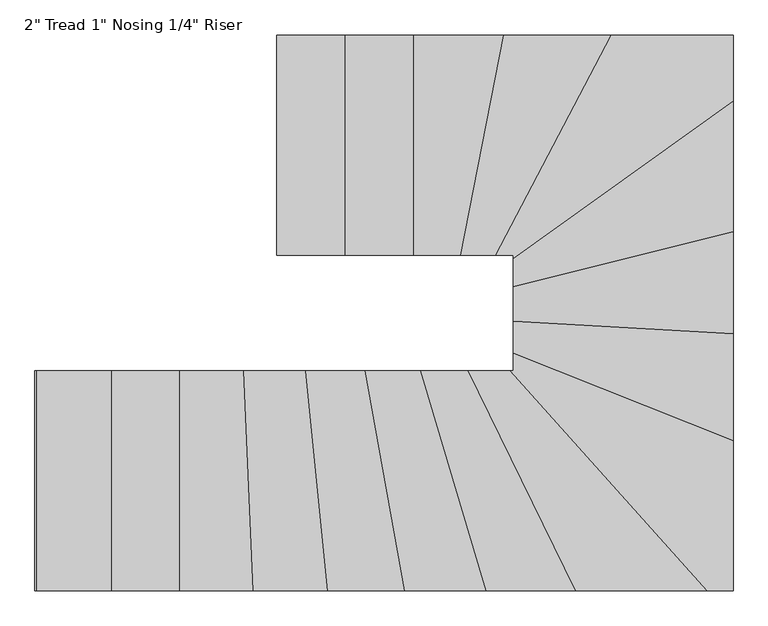
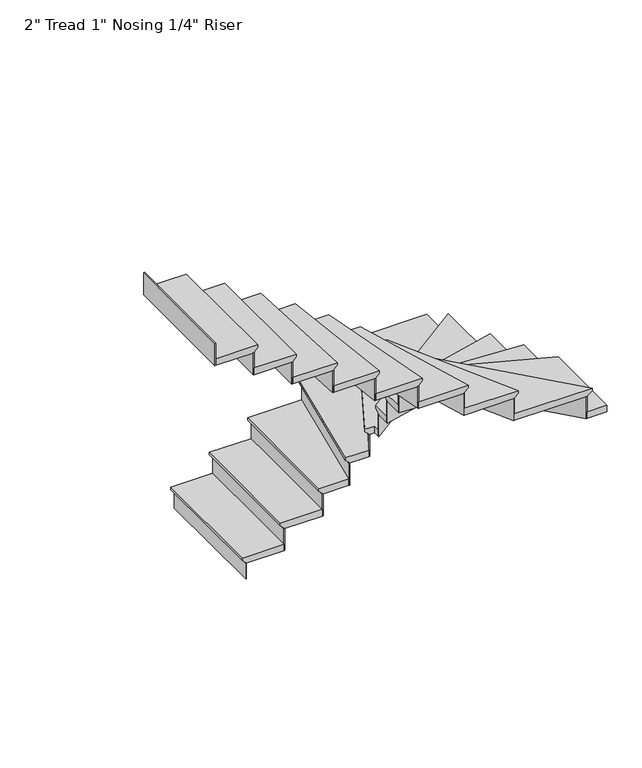
"""IFC4 building model written with IfcOpenShell, lengths in millimetres: stair flight geometry."""

from ifc_helpers import new_model, si_unit, origin, place, context, project, spatial, faceted_brep, source, transform, mapped, element, save


def stair_flight_546a6d32(model_context):
    return source(origin(), model_context, "Body", "Brep", [
        faceted_brep([(158.6923968, 2024.0935985, 3350.6833333), (158.6923968, 2024.0935985, 3369.7333333), (158.6923968, 2922.8476133, 3369.7333333), (158.6923968, 2922.8476133, 3350.6833333), (184.0923968, 2024.0935985, 3325.2833333), (184.0923968, 2922.8476133, 3325.2833333), (463.4923968, 2024.0935985, 3369.7333333), (463.4923968, 2922.8476133, 3369.7333333), (184.0923968, 2922.8476133, 3318.9333333), (463.4923968, 2922.8476133, 3318.9333333), (463.4923968, 2024.0935985, 3318.9333333), (184.0923968, 2024.0935985, 3318.9333333)], [[[0, 1, 2, 3]], [[4, 0, 3, 5]], [[2, 1, 6, 7]], [[8, 9, 10, 11]], [[2, 7, 9, 8, 5, 3]], [[8, 11, 4, 5]], [[6, 1, 0, 4, 11, 10]], [[7, 6, 10, 9]]]),
        faceted_brep([(184.0923968, 2024.0935985, 3318.9333333), (184.0923968, 2024.0935985, 3200.4), (190.4423968, 2024.0935985, 3200.4), (190.4423968, 2024.0935985, 3318.9333333), (184.0923968, 2922.8476133, 3318.9333333), (190.4423968, 2922.8476133, 3318.9333333), (190.4423968, 2922.8476133, 3200.4), (184.0923968, 2922.8476133, 3200.4)], [[[0, 1, 2, 3]], [[4, 5, 6, 7]], [[1, 0, 4, 7]], [[2, 1, 7, 6]], [[3, 2, 6, 5]], [[0, 3, 5, 4]]]),
        faceted_brep([(463.4923968, 2024.0935985, 3488.2666667), (463.4923968, 2024.0935985, 3318.9333333), (469.8423968, 2024.0935985, 3318.9333333), (469.8423968, 2024.0935985, 3488.2666667), (463.4923968, 2922.8476133, 3488.2666667), (469.8423968, 2922.8476133, 3488.2666667), (469.8423968, 2922.8476133, 3318.9333333), (463.4923968, 2922.8476133, 3318.9333333)], [[[0, 1, 2, 3]], [[4, 5, 6, 7]], [[1, 0, 4, 7]], [[2, 1, 7, 6]], [[3, 2, 6, 5]], [[0, 3, 5, 4]]]),
        faceted_brep([(438.0923968, 2922.8476133, 3539.0666667), (438.0923968, 2024.0935985, 3539.0666667), (742.8923968, 2024.0935985, 3539.0666667), (742.8923968, 2922.8476133, 3539.0666667), (463.4923968, 2922.8476133, 3488.2666667), (742.8923968, 2922.8476133, 3488.2666667), (742.8923968, 2024.0935985, 3488.2666667), (463.4923968, 2024.0935985, 3488.2666667), (463.4923968, 2922.8476133, 3494.6166667), (438.0923968, 2922.8476133, 3520.0166667), (463.4923968, 2024.0935985, 3494.6166667), (438.0923968, 2024.0935985, 3520.0166667)], [[[0, 1, 2, 3]], [[4, 5, 6, 7]], [[0, 3, 5, 4, 8, 9]], [[4, 7, 10, 8]], [[2, 1, 11, 10, 7, 6]], [[3, 2, 6, 5]], [[11, 1, 0, 9]], [[10, 11, 9, 8]]]),
        faceted_brep([(742.8923968, 2024.0935985, 3657.6), (742.8923968, 2024.0935985, 3488.2666667), (749.2423968, 2024.0935985, 3488.2666667), (749.2423968, 2024.0935985, 3657.6), (742.8923968, 2922.8476133, 3657.6), (749.2423968, 2922.8476133, 3657.6), (749.2423968, 2922.8476133, 3488.2666667), (742.8923968, 2922.8476133, 3488.2666667)], [[[0, 1, 2, 3]], [[4, 5, 6, 7]], [[1, 0, 4, 7]], [[2, 1, 7, 6]], [[3, 2, 6, 5]], [[0, 3, 5, 4]]]),
        faceted_brep([(717.4923968, 2922.8476133, 3708.4), (717.4923968, 2024.0935985, 3708.4), (934.4682952, 2024.0935985, 3708.4), (1111.0881205, 2922.8476133, 3708.4), (742.8923968, 2922.8476133, 3657.6), (1111.0881205, 2922.8476133, 3657.6), (934.4682952, 2024.0935985, 3657.6), (742.8923968, 2024.0935985, 3657.6), (742.8923968, 2922.8476133, 3663.95), (717.4923968, 2922.8476133, 3689.35), (742.8923968, 2024.0935985, 3663.95), (717.4923968, 2024.0935985, 3689.35)], [[[0, 1, 2, 3]], [[4, 5, 6, 7]], [[0, 3, 5, 4, 8, 9]], [[4, 7, 10, 8]], [[2, 1, 11, 10, 7, 6]], [[3, 2, 6, 5]], [[11, 1, 0, 9]], [[10, 11, 9, 8]]]),
        faceted_brep([(934.4682952, 2024.0935985, 3826.9333333), (934.4682952, 2024.0935985, 3657.6), (940.939748, 2024.0935985, 3657.6), (940.939748, 2024.0935985, 3826.9333333), (1111.0881205, 2922.8476133, 3826.9333333), (1117.5595733, 2922.8476133, 3826.9333333), (1117.5595733, 2922.8476133, 3657.6), (1111.0881205, 2922.8476133, 3657.6)], [[[0, 1, 2, 3]], [[4, 5, 6, 7]], [[1, 0, 4, 7]], [[2, 1, 7, 6]], [[3, 2, 6, 5]], [[0, 3, 5, 4]]]),
        faceted_brep([(1085.2023094, 2922.8476133, 3877.7333333), (908.5824841, 2024.0935985, 3877.7333333), (1081.601446, 2024.0935985, 3877.7333333), (1553.5566487, 2922.8476133, 3877.7333333), (1111.0881205, 2922.8476133, 3826.9333333), (1553.5566487, 2922.8476133, 3826.9333333), (1081.601446, 2024.0935985, 3826.9333333), (934.4682952, 2024.0935985, 3826.9333333), (1111.0881205, 2922.8476133, 3833.2833333), (1085.2023094, 2922.8476133, 3858.6833333), (934.4682952, 2024.0935985, 3833.2833333), (908.5824841, 2024.0935985, 3858.6833333)], [[[0, 1, 2, 3]], [[4, 5, 6, 7]], [[0, 3, 5, 4, 8, 9]], [[4, 7, 10, 8]], [[2, 1, 11, 10, 7, 6]], [[3, 2, 6, 5]], [[11, 1, 0, 9]], [[10, 11, 9, 8]]]),
        faceted_brep([(1081.601446, 2024.0935985, 3996.2666667), (1081.601446, 2024.0935985, 3826.9333333), (1088.7737218, 2024.0935985, 3826.9333333), (1088.7737218, 2024.0935985, 3996.2666667), (1553.5566487, 2922.8476133, 3996.2666667), (1560.7289245, 2922.8476133, 3996.2666667), (1560.7289245, 2922.8476133, 3826.9333333), (1553.5566487, 2922.8476133, 3826.9333333)], [[[0, 1, 2, 3]], [[4, 5, 6, 7]], [[1, 0, 4, 7]], [[2, 1, 7, 6]], [[3, 2, 6, 5]], [[0, 3, 5, 4]]]),
        faceted_brep([(2022.1441983, 2621.1058304, 4047.0666667), (2022.1441983, 2922.8476133, 4047.0666667), (1524.8675453, 2922.8476133, 4047.0666667), (1052.9123426, 2024.0935985, 4047.0666667), (1123.3901835, 2024.0935985, 4047.0666667), (1123.3901835, 1978.1363323, 4047.0666667), (2022.1441983, 2922.8476133, 3996.2666667), (2022.1441983, 2621.1058304, 3996.2666667), (1123.3901835, 1978.1363323, 3996.2666667), (1123.3901835, 2024.0935985, 3996.2666667), (1081.601446, 2024.0935985, 3996.2666667), (1553.5566487, 2922.8476133, 3996.2666667), (1081.601446, 2024.0935985, 4002.6166667), (1553.5566487, 2922.8476133, 4002.6166667), (1052.9123426, 2024.0935985, 4028.0166667), (1524.8675453, 2922.8476133, 4028.0166667)], [[[0, 1, 2, 3, 4, 5]], [[6, 7, 8, 9, 10, 11]], [[1, 0, 7, 6]], [[11, 10, 12, 13]], [[4, 3, 14, 12, 10, 9]], [[0, 5, 8, 7]], [[14, 3, 2, 15]], [[12, 14, 15, 13]], [[5, 4, 9, 8]], [[2, 1, 6, 11, 13, 15]]]),
        faceted_brep([(1123.3901835, 1978.1363323, 4165.6), (1123.3901835, 1978.1363323, 3996.2666667), (1123.3901835, 1970.328676, 3996.2666667), (1123.3901835, 1970.328676, 4165.6), (2022.1441983, 2621.1058304, 4165.6), (2022.1441983, 2613.298174, 4165.6), (2022.1441983, 2613.298174, 3996.2666667), (2022.1441983, 2621.1058304, 3996.2666667)], [[[0, 1, 2, 3]], [[4, 5, 6, 7]], [[1, 0, 4, 7]], [[2, 1, 7, 6]], [[3, 2, 6, 5]], [[0, 3, 5, 4]]]),
        faceted_brep([(2022.1441983, 2652.3364556, 4216.4), (1123.3901835, 2009.3669576, 4216.4), (1123.3901835, 1868.1880985, 4216.4), (2022.1441983, 2093.75794, 4216.4), (2022.1441983, 2621.1058304, 4165.6), (2022.1441983, 2093.75794, 4165.6), (1123.3901835, 1868.1880985, 4165.6), (1123.3901835, 1978.1363323, 4165.6), (2022.1441983, 2621.1058304, 4171.95), (2022.1441983, 2652.3364556, 4197.35), (1123.3901835, 1978.1363323, 4171.95), (1123.3901835, 2009.3669576, 4197.35)], [[[0, 1, 2, 3]], [[4, 5, 6, 7]], [[0, 3, 5, 4, 8, 9]], [[4, 7, 10, 8]], [[2, 1, 11, 10, 7, 6]], [[3, 2, 6, 5]], [[11, 1, 0, 9]], [[10, 11, 9, 8]]]),
        faceted_brep([(1123.3901835, 1868.1880985, 4334.9333333), (1123.3901835, 1868.1880985, 4165.6), (1123.3901835, 1861.6411553, 4165.6), (1123.3901835, 1861.6411553, 4334.9333333), (2022.1441983, 2093.75794, 4334.9333333), (2022.1441983, 2087.2109968, 4334.9333333), (2022.1441983, 2087.2109968, 4165.6), (2022.1441983, 2093.75794, 4165.6)], [[[0, 1, 2, 3]], [[4, 5, 6, 7]], [[1, 0, 4, 7]], [[2, 1, 7, 6]], [[3, 2, 6, 5]], [[0, 3, 5, 4]]]),
        faceted_brep([(2022.1441983, 2119.9457129, 4385.7333333), (1123.3901835, 1894.3758714, 4385.7333333), (1123.3901835, 1727.7101185, 4385.7333333), (2022.1441983, 1676.930447, 4385.7333333), (2022.1441983, 2093.75794, 4334.9333333), (2022.1441983, 1676.930447, 4334.9333333), (1123.3901835, 1727.7101185, 4334.9333333), (1123.3901835, 1868.1880985, 4334.9333333), (2022.1441983, 2093.75794, 4341.2833333), (2022.1441983, 2119.9457129, 4366.6833333), (1123.3901835, 1868.1880985, 4341.2833333), (1123.3901835, 1894.3758714, 4366.6833333)], [[[0, 1, 2, 3]], [[4, 5, 6, 7]], [[0, 3, 5, 4, 8, 9]], [[4, 7, 10, 8]], [[2, 1, 11, 10, 7, 6]], [[3, 2, 6, 5]], [[11, 1, 0, 9]], [[10, 11, 9, 8]]]),
        faceted_brep([(1123.3901835, 1727.7101185, 4504.2666667), (1123.3901835, 1727.7101185, 4334.9333333), (1123.3901835, 1721.3499912, 4334.9333333), (1123.3901835, 1721.3499912, 4504.2666667), (2022.1441983, 1676.930447, 4504.2666667), (2022.1441983, 1670.5703197, 4504.2666667), (2022.1441983, 1670.5703197, 4334.9333333), (2022.1441983, 1676.930447, 4334.9333333)], [[[0, 1, 2, 3]], [[4, 5, 6, 7]], [[1, 0, 4, 7]], [[2, 1, 7, 6]], [[3, 2, 6, 5]], [[0, 3, 5, 4]]]),
        faceted_brep([(2022.1441983, 1702.3709564, 4555.0666667), (1123.3901835, 1753.1506279, 4555.0666667), (1123.3901835, 1594.7393557, 4555.0666667), (2022.1441983, 1238.4229709, 4555.0666667), (2022.1441983, 1676.930447, 4504.2666667), (2022.1441983, 1238.4229709, 4504.2666667), (1123.3901835, 1594.7393557, 4504.2666667), (1123.3901835, 1727.7101185, 4504.2666667), (2022.1441983, 1676.930447, 4510.6166667), (2022.1441983, 1702.3709564, 4536.0166667), (1123.3901835, 1727.7101185, 4510.6166667), (1123.3901835, 1753.1506279, 4536.0166667)], [[[0, 1, 2, 3]], [[4, 5, 6, 7]], [[0, 3, 5, 4, 8, 9]], [[4, 7, 10, 8]], [[3, 2, 6, 5]], [[11, 1, 0, 9]], [[10, 11, 9, 8]], [[2, 1, 11, 10, 7, 6]]]),
        faceted_brep([(1123.3901835, 1594.7393557, 4673.6), (1123.3901835, 1594.7393557, 4504.2666667), (1123.3901835, 1587.9085225, 4504.2666667), (1123.3901835, 1587.9085225, 4673.6), (2022.1441983, 1238.4229709, 4673.6), (2022.1441983, 1231.5921376, 4673.6), (2022.1441983, 1231.5921376, 4504.2666667), (2022.1441983, 1238.4229709, 4504.2666667)], [[[0, 1, 2, 3]], [[4, 5, 6, 7]], [[1, 0, 4, 7]], [[2, 1, 7, 6]], [[3, 2, 6, 5]], [[0, 3, 5, 4]]]),
        faceted_brep([(1880.1651285, 652.4935985, 4724.4), (2022.1441983, 652.4935985, 4724.4), (2022.1441983, 1265.7463038, 4724.4), (1123.3901835, 1622.0626887, 4724.4), (1123.3901835, 1551.2476133, 4724.4), (1076.3040211, 1551.2476133, 4724.4), (2022.1441983, 652.4935985, 4673.6), (1880.1651285, 652.4935985, 4673.6), (1076.3040211, 1551.2476133, 4673.6), (1123.3901835, 1551.2476133, 4673.6), (1123.3901835, 1594.7393557, 4673.6), (2022.1441983, 1238.4229709, 4673.6), (1123.3901835, 1594.7393557, 4679.95), (2022.1441983, 1238.4229709, 4679.95), (1123.3901835, 1622.0626887, 4705.35), (2022.1441983, 1265.7463038, 4705.35)], [[[0, 1, 2, 3, 4, 5]], [[6, 7, 8, 9, 10, 11]], [[1, 0, 7, 6]], [[11, 10, 12, 13]], [[4, 3, 14, 12, 10, 9]], [[0, 5, 8, 7]], [[14, 3, 2, 15]], [[12, 14, 15, 13]], [[2, 1, 6, 11, 13, 15]], [[5, 4, 9, 8]]]),
        faceted_brep([(1076.3040211, 1551.2476133, 4842.9333333), (1076.3040211, 1551.2476133, 4673.6), (1067.7846442, 1551.2476133, 4673.6), (1067.7846442, 1551.2476133, 4842.9333333), (1880.1651285, 652.4935985, 4842.9333333), (1871.6457515, 652.4935985, 4842.9333333), (1871.6457515, 652.4935985, 4673.6), (1880.1651285, 652.4935985, 4673.6)], [[[0, 1, 2, 3]], [[4, 5, 6, 7]], [[1, 0, 4, 7]], [[2, 1, 7, 6]], [[3, 2, 6, 5]], [[0, 3, 5, 4]]]),
        faceted_brep([(1914.2426364, 652.4935985, 4893.7333333), (1110.381529, 1551.2476133, 4893.7333333), (909.9761874, 1551.2476133, 4893.7333333), (1349.6820711, 652.4935985, 4893.7333333), (1880.1651285, 652.4935985, 4842.9333333), (1349.6820711, 652.4935985, 4842.9333333), (909.9761874, 1551.2476133, 4842.9333333), (1076.3040211, 1551.2476133, 4842.9333333), (1880.1651285, 652.4935985, 4849.2833333), (1914.2426364, 652.4935985, 4874.6833333), (1076.3040211, 1551.2476133, 4849.2833333), (1110.381529, 1551.2476133, 4874.6833333)], [[[0, 1, 2, 3]], [[4, 5, 6, 7]], [[0, 3, 5, 4, 8, 9]], [[4, 7, 10, 8]], [[2, 1, 11, 10, 7, 6]], [[3, 2, 6, 5]], [[11, 1, 0, 9]], [[10, 11, 9, 8]]]),
        faceted_brep([(909.9761874, 1551.2476133, 5012.2666667), (909.9761874, 1551.2476133, 4842.9333333), (902.9069653, 1551.2476133, 4842.9333333), (902.9069653, 1551.2476133, 5012.2666667), (1349.6820711, 652.4935985, 5012.2666667), (1342.6128491, 652.4935985, 5012.2666667), (1342.6128491, 652.4935985, 4842.9333333), (1349.6820711, 652.4935985, 4842.9333333)], [[[0, 1, 2, 3]], [[4, 5, 6, 7]], [[1, 0, 4, 7]], [[2, 1, 7, 6]], [[3, 2, 6, 5]], [[0, 3, 5, 4]]]),
        faceted_brep([(1377.9589592, 652.4935985, 5063.0666667), (938.2530755, 1551.2476133, 5063.0666667), (717.8211109, 1551.2476133, 5063.0666667), (985.3279709, 652.4935985, 5063.0666667), (1349.6820711, 652.4935985, 5012.2666667), (985.3279709, 652.4935985, 5012.2666667), (717.8211109, 1551.2476133, 5012.2666667), (909.9761874, 1551.2476133, 5012.2666667), (1349.6820711, 652.4935985, 5018.6166667), (1377.9589592, 652.4935985, 5044.0166667), (909.9761874, 1551.2476133, 5018.6166667), (938.2530755, 1551.2476133, 5044.0166667)], [[[0, 1, 2, 3]], [[4, 5, 6, 7]], [[0, 3, 5, 4, 8, 9]], [[4, 7, 10, 8]], [[2, 1, 11, 10, 7, 6]], [[3, 2, 6, 5]], [[11, 1, 0, 9]], [[10, 11, 9, 8]]]),
        faceted_brep([(717.8211109, 1551.2476133, 5181.6), (717.8211109, 1551.2476133, 5012.2666667), (711.1958034, 1551.2476133, 5012.2666667), (711.1958034, 1551.2476133, 5181.6), (985.3279709, 652.4935985, 5181.6), (978.7026634, 652.4935985, 5181.6), (978.7026634, 652.4935985, 5012.2666667), (985.3279709, 652.4935985, 5012.2666667)], [[[0, 1, 2, 3]], [[4, 5, 6, 7]], [[1, 0, 4, 7]], [[2, 1, 7, 6]], [[3, 2, 6, 5]], [[0, 3, 5, 4]]]),
        faceted_brep([(1011.8292006, 652.4935985, 5232.4), (744.3223406, 1551.2476133, 5232.4), (491.9145253, 1551.2476133, 5232.4), (653.8193232, 652.4935985, 5232.4), (985.3279709, 652.4935985, 5181.6), (653.8193232, 652.4935985, 5181.6), (491.9145253, 1551.2476133, 5181.6), (717.8211109, 1551.2476133, 5181.6), (985.3279709, 652.4935985, 5187.95), (1011.8292006, 652.4935985, 5213.35), (717.8211109, 1551.2476133, 5187.95), (744.3223406, 1551.2476133, 5213.35)], [[[0, 1, 2, 3]], [[4, 5, 6, 7]], [[0, 3, 5, 4, 8, 9]], [[4, 7, 10, 8]], [[2, 1, 11, 10, 7, 6]], [[3, 2, 6, 5]], [[11, 1, 0, 9]], [[10, 11, 9, 8]]]),
        faceted_brep([(491.9145253, 1551.2476133, 5350.9333333), (491.9145253, 1551.2476133, 5181.6), (485.4623137, 1551.2476133, 5181.6), (485.4623137, 1551.2476133, 5350.9333333), (653.8193232, 652.4935985, 5350.9333333), (647.3671116, 652.4935985, 5350.9333333), (647.3671116, 652.4935985, 5181.6), (653.8193232, 652.4935985, 5181.6)], [[[0, 1, 2, 3]], [[4, 5, 6, 7]], [[1, 0, 4, 7]], [[2, 1, 7, 6]], [[3, 2, 6, 5]], [[0, 3, 5, 4]]]),
        faceted_brep([(679.6281696, 652.4935985, 5401.7333333), (517.7233717, 1551.2476133, 5401.7333333), (248.510664, 1551.2476133, 5401.7333333), (338.9841344, 652.4935985, 5401.7333333), (653.8193232, 652.4935985, 5350.9333333), (338.9841344, 652.4935985, 5350.9333333), (248.510664, 1551.2476133, 5350.9333333), (491.9145253, 1551.2476133, 5350.9333333), (653.8193232, 652.4935985, 5357.2833333), (679.6281696, 652.4935985, 5382.6833333), (491.9145253, 1551.2476133, 5357.2833333), (517.7233717, 1551.2476133, 5382.6833333)], [[[0, 1, 2, 3]], [[4, 5, 6, 7]], [[0, 3, 5, 4, 8, 9]], [[4, 7, 10, 8]], [[2, 1, 11, 10, 7, 6]], [[3, 2, 6, 5]], [[11, 1, 0, 9]], [[10, 11, 9, 8]]]),
        faceted_brep([(248.510664, 1551.2476133, 5520.2666667), (248.510664, 1551.2476133, 5350.9333333), (242.1285711, 1551.2476133, 5350.9333333), (242.1285711, 1551.2476133, 5520.2666667), (338.9841344, 652.4935985, 5520.2666667), (332.6020415, 652.4935985, 5520.2666667), (332.6020415, 652.4935985, 5350.9333333), (338.9841344, 652.4935985, 5350.9333333)], [[[0, 1, 2, 3]], [[4, 5, 6, 7]], [[1, 0, 4, 7]], [[2, 1, 7, 6]], [[3, 2, 6, 5]], [[0, 3, 5, 4]]]),
        faceted_brep([(364.5125059, 652.4935985, 5571.0666667), (274.0390354, 1551.2476133, 5571.0666667), (-5.0166043, 1551.2476133, 5571.0666667), (33.9204942, 652.4935985, 5571.0666667), (338.9841344, 652.4935985, 5520.2666667), (33.9204942, 652.4935985, 5520.2666667), (-5.0166043, 1551.2476133, 5520.2666667), (248.510664, 1551.2476133, 5520.2666667), (338.9841344, 652.4935985, 5526.6166667), (364.5125059, 652.4935985, 5552.0166667), (248.510664, 1551.2476133, 5526.6166667), (274.0390354, 1551.2476133, 5552.0166667)], [[[0, 1, 2, 3]], [[4, 5, 6, 7]], [[0, 3, 5, 4, 8, 9]], [[4, 7, 10, 8]], [[2, 1, 11, 10, 7, 6]], [[3, 2, 6, 5]], [[11, 1, 0, 9]], [[10, 11, 9, 8]]]),
        faceted_brep([(-5.0166043, 1551.2476133, 5689.6), (-5.0166043, 1551.2476133, 5520.2666667), (-11.3725607, 1551.2476133, 5520.2666667), (-11.3725607, 1551.2476133, 5689.6), (33.9204942, 652.4935985, 5689.6), (27.5645378, 652.4935985, 5689.6), (27.5645378, 652.4935985, 5520.2666667), (33.9204942, 652.4935985, 5520.2666667)], [[[0, 1, 2, 3]], [[4, 5, 6, 7]], [[1, 0, 4, 7]], [[2, 1, 7, 6]], [[3, 2, 6, 5]], [[0, 3, 5, 4]]]),
        faceted_brep([(59.3443199, 652.4935985, 5740.4), (20.4072214, 1551.2476133, 5740.4), (-264.9242294, 1551.2476133, 5740.4), (-264.9242294, 652.4935985, 5740.4), (33.9204942, 652.4935985, 5689.6), (-264.9242294, 652.4935985, 5689.6), (-264.9242294, 1551.2476133, 5689.6), (-5.0166043, 1551.2476133, 5689.6), (33.9204942, 652.4935985, 5695.95), (59.3443199, 652.4935985, 5721.35), (-5.0166043, 1551.2476133, 5695.95), (20.4072214, 1551.2476133, 5721.35)], [[[0, 1, 2, 3]], [[4, 5, 6, 7]], [[0, 3, 5, 4, 8, 9]], [[4, 7, 10, 8]], [[2, 1, 11, 10, 7, 6]], [[3, 2, 6, 5]], [[11, 1, 0, 9]], [[10, 11, 9, 8]]]),
        faceted_brep([(-264.9242294, 1551.2476133, 5858.9333333), (-264.9242294, 1551.2476133, 5689.6), (-271.2742294, 1551.2476133, 5689.6), (-271.2742294, 1551.2476133, 5858.9333333), (-264.9242294, 652.4935985, 5858.9333333), (-271.2742294, 652.4935985, 5858.9333333), (-271.2742294, 652.4935985, 5689.6), (-264.9242294, 652.4935985, 5689.6)], [[[0, 1, 2, 3]], [[4, 5, 6, 7]], [[1, 0, 4, 7]], [[2, 1, 7, 6]], [[3, 2, 6, 5]], [[0, 3, 5, 4]]]),
        faceted_brep([(-239.5242294, 652.4935985, 5909.7333333), (-239.5242294, 1551.2476133, 5909.7333333), (-544.3242294, 1551.2476133, 5909.7333333), (-544.3242294, 652.4935985, 5909.7333333), (-264.9242294, 652.4935985, 5858.9333333), (-544.3242294, 652.4935985, 5858.9333333), (-544.3242294, 1551.2476133, 5858.9333333), (-264.9242294, 1551.2476133, 5858.9333333), (-264.9242294, 652.4935985, 5865.2833333), (-239.5242294, 652.4935985, 5890.6833333), (-264.9242294, 1551.2476133, 5865.2833333), (-239.5242294, 1551.2476133, 5890.6833333)], [[[0, 1, 2, 3]], [[4, 5, 6, 7]], [[0, 3, 5, 4, 8, 9]], [[4, 7, 10, 8]], [[2, 1, 11, 10, 7, 6]], [[3, 2, 6, 5]], [[11, 1, 0, 9]], [[10, 11, 9, 8]]]),
        faceted_brep([(-544.3242294, 1551.2476133, 6028.2666667), (-544.3242294, 1551.2476133, 5858.9333333), (-550.6742294, 1551.2476133, 5858.9333333), (-550.6742294, 1551.2476133, 6028.2666667), (-544.3242294, 652.4935985, 6028.2666667), (-550.6742294, 652.4935985, 6028.2666667), (-550.6742294, 652.4935985, 5858.9333333), (-544.3242294, 652.4935985, 5858.9333333)], [[[0, 1, 2, 3]], [[4, 5, 6, 7]], [[1, 0, 4, 7]], [[2, 1, 7, 6]], [[3, 2, 6, 5]], [[0, 3, 5, 4]]]),
        faceted_brep([(-823.7242294, 1551.2476133, 6197.6), (-823.7242294, 1551.2476133, 6028.2666667), (-830.0742294, 1551.2476133, 6028.2666667), (-830.0742294, 1551.2476133, 6197.6), (-823.7242294, 652.4935985, 6197.6), (-830.0742294, 652.4935985, 6197.6), (-830.0742294, 652.4935985, 6028.2666667), (-823.7242294, 652.4935985, 6028.2666667)], [[[0, 1, 2, 3]], [[4, 5, 6, 7]], [[1, 0, 4, 7]], [[2, 1, 7, 6]], [[3, 2, 6, 5]], [[0, 3, 5, 4]]]),
        faceted_brep([(-518.9242294, 652.4935985, 6079.0666667), (-518.9242294, 1551.2476133, 6079.0666667), (-823.7242294, 1551.2476133, 6079.0666667), (-823.7242294, 652.4935985, 6079.0666667), (-544.3242294, 652.4935985, 6028.2666667), (-823.7242294, 652.4935985, 6028.2666667), (-823.7242294, 1551.2476133, 6028.2666667), (-544.3242294, 1551.2476133, 6028.2666667), (-544.3242294, 652.4935985, 6034.6166667), (-518.9242294, 652.4935985, 6060.0166667), (-544.3242294, 1551.2476133, 6034.6166667), (-518.9242294, 1551.2476133, 6060.0166667)], [[[0, 1, 2, 3]], [[4, 5, 6, 7]], [[0, 3, 5, 4, 8, 9]], [[4, 7, 10, 8]], [[2, 1, 11, 10, 7, 6]], [[3, 2, 6, 5]], [[11, 1, 0, 9]], [[10, 11, 9, 8]]]),
    ])


if __name__ == "__main__":
    model = new_model("IFC4")
    model_context = context("Model", 3, world=origin())
    ifc_project = project(units=[si_unit("LENGTHUNIT", "METRE", prefix="MILLI")], contexts=[model_context])
    site = spatial("IfcSite", under=ifc_project)
    building = spatial("IfcBuilding", under=site)
    placement = place(None, origin())
    stair_flight_shape = stair_flight_546a6d32(model_context)
    element("IfcStairFlight", 1, ObjectType="2\" Tread 1\" Nosing 1/4\" Riser", at=placement, inside=building, context=model_context, shape_type="MappedRepresentation", body=[
        mapped(stair_flight_shape, transform((0.0, 0.0, 0.0), x_axis=(1.0, 0.0, 0.0), y_axis=(0.0, 1.0, 0.0), z_axis=(0.0, 0.0, 1.0))),
    ])
    save(model, "model.ifc")
